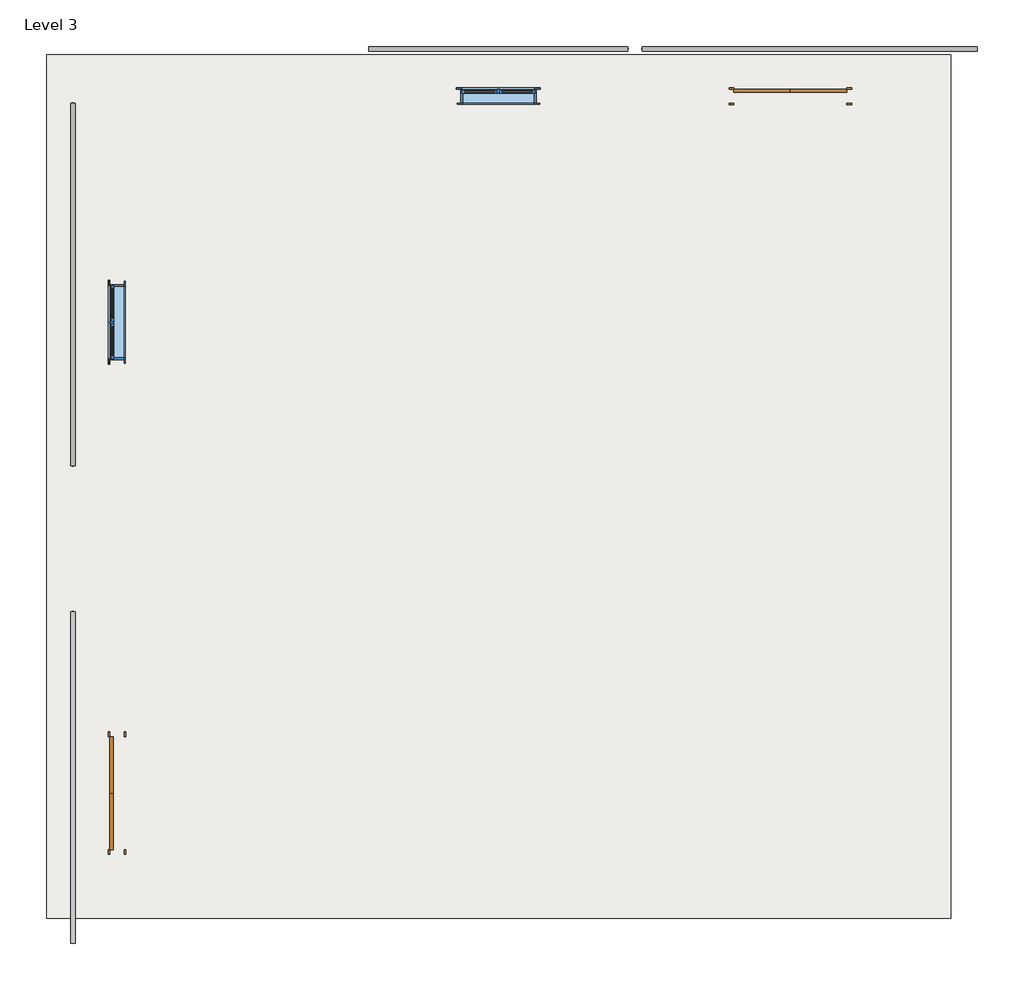
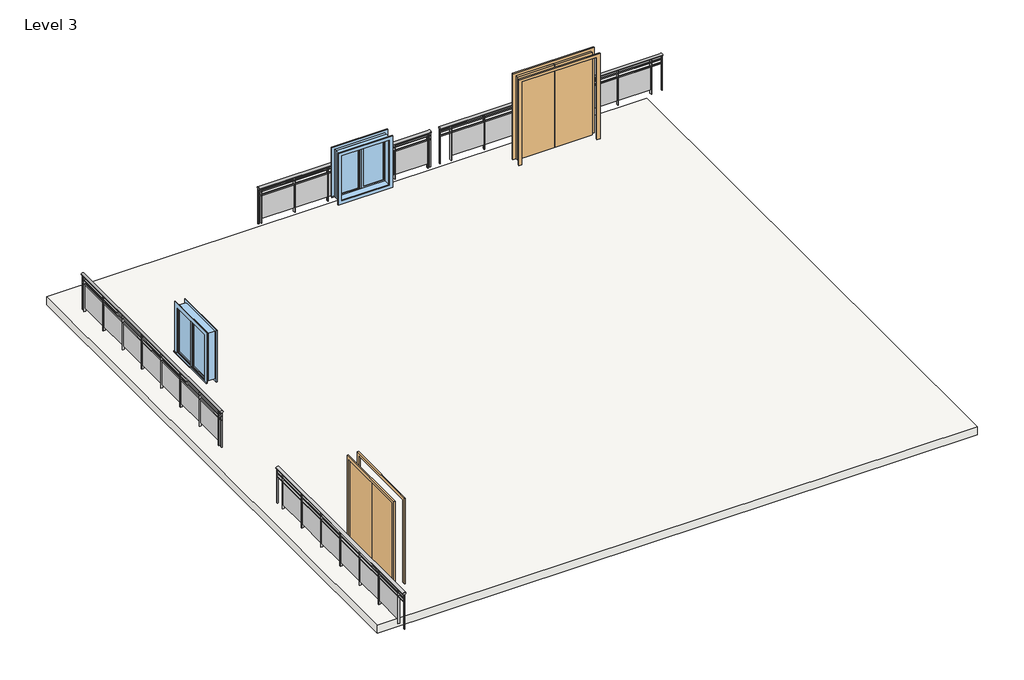
# One storey: 4 railings, 2 doors, 2 windows, 1 slab.
"""IFC4 building model written with IfcOpenShell, lengths in millimetres."""

from ifc_helpers import new_model, si_unit, point, frame, origin, place, context, project, spatial, polyline, ellipse_curve, trimmed, outline, extrude, transform, mapped, element, save
from ifc_brep_helpers import plane_surface, extruded_surface, advanced_brep
from components import door_640b4634, window_534dcd48

model = new_model("IFC4")

# Units and contexts
model_context = context("Model", 3, world=origin())
ifc_project = project(units=[si_unit("LENGTHUNIT", "METRE", prefix="MILLI")], contexts=[model_context])

# Site, building, storey
site = spatial("IfcSite", under=ifc_project)
building = spatial("IfcBuilding", under=site)
storey = spatial("IfcBuildingStorey", under=building, Name="Level 3", Elevation=6400.8)

# Doors
placement = place(None, origin())
door_shape = door_640b4634(model_context)
element("IfcDoor", 1, ObjectType="Door-Double-Flush_Panel : 72\" x 84\"", at=placement, inside=storey, context=model_context, shape_type="MappedRepresentation", body=[
    mapped(door_shape, transform((-18468.543393, -7089.1397804, 6400.8), x_axis=(0.0, 1.0, 0.0), y_axis=(-1.0, 0.0, 0.0), z_axis=(0.0, 0.0, 1.0))),
])
element("IfcDoor", 2, ObjectType="Door-Double-Flush_Panel : 72\" x 84\"", at=placement, inside=storey, context=model_context, shape_type="MappedRepresentation", body=[
    mapped(door_shape, transform((-7571.943393, 4188.4602196, 6400.8), x_axis=(1.0, 0.0, 0.0), y_axis=(0.0, 1.0, 0.0), z_axis=(0.0, 0.0, 1.0))),
])

# Railings
element("IfcRailing", 3, ObjectType="Glass Panel - Bottom Fill", at=placement, inside=storey, context=model_context, shape_type="SolidModel", body=[
    advanced_brep(
    [(-19220.0296876, -9514.8397804, 7315.2), (-19143.8296876, -9514.8397804, 7315.2), (-19220.0296876, -4155.4397804, 7315.2), (-19143.8296876, -4155.4397804, 7315.2)],
    [
        (0, 1, ellipse_curve(frame((-19181.9296876, -9514.8397804, 7315.2), z_axis=(0.0, -1.0, 0.0), x_axis=(1.0, 0.0, 0.0)), 38.1, 28.575)),
        (1, 0, ellipse_curve(frame((-19181.9296876, -9514.8397804, 7315.2), z_axis=(0.0, -1.0, 0.0), x_axis=(1.0, 0.0, 0.0)), 38.1, 28.575)),
        (2, 3, ellipse_curve(frame((-19181.9296876, -4155.4397804, 7315.2), z_axis=(0.0, 1.0, 0.0), x_axis=(1.0, 0.0, 0.0)), 38.1, 28.575)),
        (3, 2, ellipse_curve(frame((-19181.9296876, -4155.4397804, 7315.2), z_axis=(0.0, 1.0, 0.0), x_axis=(1.0, 0.0, 0.0)), 38.1, 28.575)),
        (0, 2),
        (3, 1),
    ],
    [
        plane_surface(frame((-19181.9296876, -9514.8397804, 7315.2), z_axis=(0.0, -1.0, 0.0), x_axis=(0.0, 0.0, 1.0))),
        plane_surface(frame((-19181.9296876, -4155.4397804, 7315.2), z_axis=(0.0, 1.0, 0.0), x_axis=(0.0, 0.0, 1.0))),
        extruded_surface(trimmed(ellipse_curve(frame((-19181.9296876, -4155.4397804, 7315.2), z_axis=(0.0, -1.0, 0.0), x_axis=(1.0, 0.0, 0.0)), 38.1, 28.575), [point((-19220.0296876, -4155.4397804, 7315.2))], [point((-19143.8296876, -4155.4397804, 7315.2))], True, "CARTESIAN"), (0.0, -5359.4, 0.0), 5359.4),
        extruded_surface(trimmed(ellipse_curve(frame((-19181.9296876, -4155.4397804, 7315.2), z_axis=(0.0, -1.0, 0.0), x_axis=(1.0, 0.0, 0.0)), 38.1, 28.575), [point((-19143.8296876, -4155.4397804, 7315.2))], [point((-19220.0296876, -4155.4397804, 7315.2))], True, "CARTESIAN"), (0.0, -5359.4, 0.0), 5359.4),
    ],
    [
        (0, [[1, 2]]),
        (1, [[3, 4]]),
        (2, [[-1, 5, -4, 6]]),
        (3, [[-2, -6, -3, -5]]),
    ],
),
    extrude(outline(polyline([(-19169.2296876, -9514.8397804), (-19194.6296876, -9514.8397804), (-19194.6296876, -4155.4397804), (-19169.2296876, -4155.4397804), (-19169.2296876, -9514.8397804)])), frame((0.0, 0.0, 7200.9), z_axis=(0.0, 0.0, 1.0), x_axis=(1.0, 0.0, 0.0)), (0.0, 0.0, 1.0), 25.4),
    extrude(outline(polyline([(-19169.2296876, -9514.8397804), (-19194.6296876, -9514.8397804), (-19194.6296876, -4155.4397804), (-19169.2296876, -4155.4397804), (-19169.2296876, -9514.8397804)])), frame((0.0, 0.0, 7099.3), z_axis=(0.0, 0.0, 1.0), x_axis=(1.0, 0.0, 0.0)), (0.0, 0.0, 1.0), 25.4),
    extrude(outline(polyline([(-19156.5296876, -4403.0897804), (-19207.3296876, -4403.0897804), (-19207.3296876, -4390.3897804), (-19156.5296876, -4390.3897804), (-19156.5296876, -4403.0897804)])), frame((0.0, 0.0, 6400.8), z_axis=(0.0, 0.0, 1.0), x_axis=(1.0, 0.0, 0.0)), (0.0, 0.0, 1.0), 885.6788223),
    extrude(outline(polyline([(-19188.4648446, -5209.5397804), (-19188.4648446, -4396.7397804), (-19182.1148446, -4396.7397804), (-19182.1148446, -5209.5397804), (-19188.4648446, -5209.5397804)])), frame((0.0, 0.0, 6502.4), z_axis=(0.0, 0.0, 1.0), x_axis=(1.0, 0.0, 0.0)), (0.0, 0.0, 1.0), 596.9),
    extrude(outline(polyline([(-19156.5296876, -5215.8897804), (-19207.3296876, -5215.8897804), (-19207.3296876, -5203.1897804), (-19156.5296876, -5203.1897804), (-19156.5296876, -5215.8897804)])), frame((0.0, 0.0, 6400.8), z_axis=(0.0, 0.0, 1.0), x_axis=(1.0, 0.0, 0.0)), (0.0, 0.0, 1.0), 885.6788223),
    extrude(outline(polyline([(-19188.4648446, -6022.3397804), (-19188.4648446, -5209.5397804), (-19182.1148446, -5209.5397804), (-19182.1148446, -6022.3397804), (-19188.4648446, -6022.3397804)])), frame((0.0, 0.0, 6502.4), z_axis=(0.0, 0.0, 1.0), x_axis=(1.0, 0.0, 0.0)), (0.0, 0.0, 1.0), 596.9),
    extrude(outline(polyline([(-19156.5296876, -6028.6897804), (-19207.3296876, -6028.6897804), (-19207.3296876, -6015.9897804), (-19156.5296876, -6015.9897804), (-19156.5296876, -6028.6897804)])), frame((0.0, 0.0, 6400.8), z_axis=(0.0, 0.0, 1.0), x_axis=(1.0, 0.0, 0.0)), (0.0, 0.0, 1.0), 885.6788223),
    extrude(outline(polyline([(-19188.4648446, -6835.1397804), (-19188.4648446, -6022.3397804), (-19182.1148446, -6022.3397804), (-19182.1148446, -6835.1397804), (-19188.4648446, -6835.1397804)])), frame((0.0, 0.0, 6502.4), z_axis=(0.0, 0.0, 1.0), x_axis=(1.0, 0.0, 0.0)), (0.0, 0.0, 1.0), 596.9),
    extrude(outline(polyline([(-19156.5296876, -6841.4897804), (-19207.3296876, -6841.4897804), (-19207.3296876, -6828.7897804), (-19156.5296876, -6828.7897804), (-19156.5296876, -6841.4897804)])), frame((0.0, 0.0, 6400.8), z_axis=(0.0, 0.0, 1.0), x_axis=(1.0, 0.0, 0.0)), (0.0, 0.0, 1.0), 885.6788223),
    extrude(outline(polyline([(-19188.4648446, -7647.9397804), (-19188.4648446, -6835.1397804), (-19182.1148446, -6835.1397804), (-19182.1148446, -7647.9397804), (-19188.4648446, -7647.9397804)])), frame((0.0, 0.0, 6502.4), z_axis=(0.0, 0.0, 1.0), x_axis=(1.0, 0.0, 0.0)), (0.0, 0.0, 1.0), 596.9),
    extrude(outline(polyline([(-19156.5296876, -7654.2897804), (-19207.3296876, -7654.2897804), (-19207.3296876, -7641.5897804), (-19156.5296876, -7641.5897804), (-19156.5296876, -7654.2897804)])), frame((0.0, 0.0, 6400.8), z_axis=(0.0, 0.0, 1.0), x_axis=(1.0, 0.0, 0.0)), (0.0, 0.0, 1.0), 885.6788223),
    extrude(outline(polyline([(-19188.4648446, -8460.7397804), (-19188.4648446, -7647.9397804), (-19182.1148446, -7647.9397804), (-19182.1148446, -8460.7397804), (-19188.4648446, -8460.7397804)])), frame((0.0, 0.0, 6502.4), z_axis=(0.0, 0.0, 1.0), x_axis=(1.0, 0.0, 0.0)), (0.0, 0.0, 1.0), 596.9),
    extrude(outline(polyline([(-19156.5296876, -8467.0897804), (-19207.3296876, -8467.0897804), (-19207.3296876, -8454.3897804), (-19156.5296876, -8454.3897804), (-19156.5296876, -8467.0897804)])), frame((0.0, 0.0, 6400.8), z_axis=(0.0, 0.0, 1.0), x_axis=(1.0, 0.0, 0.0)), (0.0, 0.0, 1.0), 885.6788223),
    extrude(outline(polyline([(-19188.4648446, -9273.5397804), (-19188.4648446, -8460.7397804), (-19182.1148446, -8460.7397804), (-19182.1148446, -9273.5397804), (-19188.4648446, -9273.5397804)])), frame((0.0, 0.0, 6502.4), z_axis=(0.0, 0.0, 1.0), x_axis=(1.0, 0.0, 0.0)), (0.0, 0.0, 1.0), 596.9),
    extrude(outline(polyline([(-19156.5296876, -9279.8897804), (-19207.3296876, -9279.8897804), (-19207.3296876, -9267.1897804), (-19156.5296876, -9267.1897804), (-19156.5296876, -9279.8897804)])), frame((0.0, 0.0, 6400.8), z_axis=(0.0, 0.0, 1.0), x_axis=(1.0, 0.0, 0.0)), (0.0, 0.0, 1.0), 885.6788223),
    extrude(outline(polyline([(-19172.4046876, -4168.1397804), (-19191.4546876, -4168.1397804), (-19191.4546876, -4149.0897804), (-19172.4046876, -4149.0897804), (-19172.4046876, -4168.1397804)])), frame((0.0, 0.0, 6400.8), z_axis=(0.0, 0.0, 1.0), x_axis=(1.0, 0.0, 0.0)), (0.0, 0.0, 1.0), 885.6788223),
    extrude(outline(polyline([(-19172.4046876, -9521.1897804), (-19191.4546876, -9521.1897804), (-19191.4546876, -9502.1397804), (-19172.4046876, -9502.1397804), (-19172.4046876, -9521.1897804)])), frame((0.0, 0.0, 6400.8), z_axis=(0.0, 0.0, 1.0), x_axis=(1.0, 0.0, 0.0)), (0.0, 0.0, 1.0), 885.6788223),
])
element("IfcRailing", 4, ObjectType="Glass Panel - Bottom Fill", at=placement, inside=storey, context=model_context, shape_type="SolidModel", body=[
    advanced_brep(
    [(-19143.8296876, 4074.1602196, 7315.2), (-19220.0296876, 4074.1602196, 7315.2), (-19143.8296876, -1793.2397804, 7315.2), (-19220.0296876, -1793.2397804, 7315.2)],
    [
        (0, 1, ellipse_curve(frame((-19181.9296876, 4074.1602196, 7315.2), z_axis=(0.0, 1.0, 0.0), x_axis=(-1.0, 0.0, 0.0)), 38.1, 28.575)),
        (1, 0, ellipse_curve(frame((-19181.9296876, 4074.1602196, 7315.2), z_axis=(0.0, 1.0, 0.0), x_axis=(-1.0, 0.0, 0.0)), 38.1, 28.575)),
        (2, 3, ellipse_curve(frame((-19181.9296876, -1793.2397804, 7315.2), z_axis=(0.0, -1.0, 0.0), x_axis=(-1.0, 0.0, 0.0)), 38.1, 28.575)),
        (3, 2, ellipse_curve(frame((-19181.9296876, -1793.2397804, 7315.2), z_axis=(0.0, -1.0, 0.0), x_axis=(-1.0, 0.0, 0.0)), 38.1, 28.575)),
        (0, 2),
        (3, 1),
    ],
    [
        plane_surface(frame((-19181.9296876, 4074.1602196, 7315.2), z_axis=(0.0, 1.0, 0.0), x_axis=(0.0, 0.0, -1.0))),
        plane_surface(frame((-19181.9296876, -1793.2397804, 7315.2), z_axis=(0.0, -1.0, 0.0), x_axis=(0.0, 0.0, -1.0))),
        extruded_surface(trimmed(ellipse_curve(frame((-19181.9296876, -1793.2397804, 7315.2), z_axis=(0.0, 1.0, 0.0), x_axis=(-1.0, 0.0, 0.0)), 38.1, 28.575), [point((-19143.8296876, -1793.2397804, 7315.2))], [point((-19220.0296876, -1793.2397804, 7315.2))], True, "CARTESIAN"), (0.0, 5867.4, 0.0), 5867.4),
        extruded_surface(trimmed(ellipse_curve(frame((-19181.9296876, -1793.2397804, 7315.2), z_axis=(0.0, 1.0, 0.0), x_axis=(-1.0, 0.0, 0.0)), 38.1, 28.575), [point((-19220.0296876, -1793.2397804, 7315.2))], [point((-19143.8296876, -1793.2397804, 7315.2))], True, "CARTESIAN"), (0.0, 5867.4, 0.0), 5867.4),
    ],
    [
        (0, [[1, 2]]),
        (1, [[3, 4]]),
        (2, [[-1, 5, -4, 6]]),
        (3, [[-2, -6, -3, -5]]),
    ],
),
    extrude(outline(polyline([(-19194.6296876, 4074.1602196), (-19169.2296876, 4074.1602196), (-19169.2296876, -1793.2397804), (-19194.6296876, -1793.2397804), (-19194.6296876, 4074.1602196)])), frame((0.0, 0.0, 7200.9), z_axis=(0.0, 0.0, 1.0), x_axis=(1.0, 0.0, 0.0)), (0.0, 0.0, 1.0), 25.4),
    extrude(outline(polyline([(-19194.6296876, 4074.1602196), (-19169.2296876, 4074.1602196), (-19169.2296876, -1793.2397804), (-19194.6296876, -1793.2397804), (-19194.6296876, 4074.1602196)])), frame((0.0, 0.0, 7099.3), z_axis=(0.0, 0.0, 1.0), x_axis=(1.0, 0.0, 0.0)), (0.0, 0.0, 1.0), 25.4),
    extrude(outline(polyline([(-19207.3296876, -1697.9897804), (-19156.5296876, -1697.9897804), (-19156.5296876, -1710.6897804), (-19207.3296876, -1710.6897804), (-19207.3296876, -1697.9897804)])), frame((0.0, 0.0, 6400.8), z_axis=(0.0, 0.0, 1.0), x_axis=(1.0, 0.0, 0.0)), (0.0, 0.0, 1.0), 885.6788223),
    extrude(outline(polyline([(-19175.3945306, -891.5397804), (-19175.3945306, -1704.3397804), (-19181.7445306, -1704.3397804), (-19181.7445306, -891.5397804), (-19175.3945306, -891.5397804)])), frame((0.0, 0.0, 6502.4), z_axis=(0.0, 0.0, 1.0), x_axis=(1.0, 0.0, 0.0)), (0.0, 0.0, 1.0), 596.9),
    extrude(outline(polyline([(-19207.3296876, -885.1897804), (-19156.5296876, -885.1897804), (-19156.5296876, -897.8897804), (-19207.3296876, -897.8897804), (-19207.3296876, -885.1897804)])), frame((0.0, 0.0, 6400.8), z_axis=(0.0, 0.0, 1.0), x_axis=(1.0, 0.0, 0.0)), (0.0, 0.0, 1.0), 885.6788223),
    extrude(outline(polyline([(-19175.3945306, -78.7397804), (-19175.3945306, -891.5397804), (-19181.7445306, -891.5397804), (-19181.7445306, -78.7397804), (-19175.3945306, -78.7397804)])), frame((0.0, 0.0, 6502.4), z_axis=(0.0, 0.0, 1.0), x_axis=(1.0, 0.0, 0.0)), (0.0, 0.0, 1.0), 596.9),
    extrude(outline(polyline([(-19207.3296876, -72.3897804), (-19156.5296876, -72.3897804), (-19156.5296876, -85.0897804), (-19207.3296876, -85.0897804), (-19207.3296876, -72.3897804)])), frame((0.0, 0.0, 6400.8), z_axis=(0.0, 0.0, 1.0), x_axis=(1.0, 0.0, 0.0)), (0.0, 0.0, 1.0), 885.6788223),
    extrude(outline(polyline([(-19175.3945306, 734.0602196), (-19175.3945306, -78.7397804), (-19181.7445306, -78.7397804), (-19181.7445306, 734.0602196), (-19175.3945306, 734.0602196)])), frame((0.0, 0.0, 6502.4), z_axis=(0.0, 0.0, 1.0), x_axis=(1.0, 0.0, 0.0)), (0.0, 0.0, 1.0), 596.9),
    extrude(outline(polyline([(-19207.3296876, 740.4102196), (-19156.5296876, 740.4102196), (-19156.5296876, 727.7102196), (-19207.3296876, 727.7102196), (-19207.3296876, 740.4102196)])), frame((0.0, 0.0, 6400.8), z_axis=(0.0, 0.0, 1.0), x_axis=(1.0, 0.0, 0.0)), (0.0, 0.0, 1.0), 885.6788223),
    extrude(outline(polyline([(-19175.3945306, 1546.8602196), (-19175.3945306, 734.0602196), (-19181.7445306, 734.0602196), (-19181.7445306, 1546.8602196), (-19175.3945306, 1546.8602196)])), frame((0.0, 0.0, 6502.4), z_axis=(0.0, 0.0, 1.0), x_axis=(1.0, 0.0, 0.0)), (0.0, 0.0, 1.0), 596.9),
    extrude(outline(polyline([(-19207.3296876, 1553.2102196), (-19156.5296876, 1553.2102196), (-19156.5296876, 1540.5102196), (-19207.3296876, 1540.5102196), (-19207.3296876, 1553.2102196)])), frame((0.0, 0.0, 6400.8), z_axis=(0.0, 0.0, 1.0), x_axis=(1.0, 0.0, 0.0)), (0.0, 0.0, 1.0), 885.6788223),
    extrude(outline(polyline([(-19175.3945306, 2359.6602196), (-19175.3945306, 1546.8602196), (-19181.7445306, 1546.8602196), (-19181.7445306, 2359.6602196), (-19175.3945306, 2359.6602196)])), frame((0.0, 0.0, 6502.4), z_axis=(0.0, 0.0, 1.0), x_axis=(1.0, 0.0, 0.0)), (0.0, 0.0, 1.0), 596.9),
    extrude(outline(polyline([(-19207.3296876, 2366.0102196), (-19156.5296876, 2366.0102196), (-19156.5296876, 2353.3102196), (-19207.3296876, 2353.3102196), (-19207.3296876, 2366.0102196)])), frame((0.0, 0.0, 6400.8), z_axis=(0.0, 0.0, 1.0), x_axis=(1.0, 0.0, 0.0)), (0.0, 0.0, 1.0), 885.6788223),
    extrude(outline(polyline([(-19175.3945306, 3172.4602196), (-19175.3945306, 2359.6602196), (-19181.7445306, 2359.6602196), (-19181.7445306, 3172.4602196), (-19175.3945306, 3172.4602196)])), frame((0.0, 0.0, 6502.4), z_axis=(0.0, 0.0, 1.0), x_axis=(1.0, 0.0, 0.0)), (0.0, 0.0, 1.0), 596.9),
    extrude(outline(polyline([(-19207.3296876, 3178.8102196), (-19156.5296876, 3178.8102196), (-19156.5296876, 3166.1102196), (-19207.3296876, 3166.1102196), (-19207.3296876, 3178.8102196)])), frame((0.0, 0.0, 6400.8), z_axis=(0.0, 0.0, 1.0), x_axis=(1.0, 0.0, 0.0)), (0.0, 0.0, 1.0), 885.6788223),
    extrude(outline(polyline([(-19175.3945306, 3985.2602196), (-19175.3945306, 3172.4602196), (-19181.7445306, 3172.4602196), (-19181.7445306, 3985.2602196), (-19175.3945306, 3985.2602196)])), frame((0.0, 0.0, 6502.4), z_axis=(0.0, 0.0, 1.0), x_axis=(1.0, 0.0, 0.0)), (0.0, 0.0, 1.0), 596.9),
    extrude(outline(polyline([(-19207.3296876, 3991.6102196), (-19156.5296876, 3991.6102196), (-19156.5296876, 3978.9102196), (-19207.3296876, 3978.9102196), (-19207.3296876, 3991.6102196)])), frame((0.0, 0.0, 6400.8), z_axis=(0.0, 0.0, 1.0), x_axis=(1.0, 0.0, 0.0)), (0.0, 0.0, 1.0), 885.6788223),
    extrude(outline(polyline([(-19191.4546876, -1780.5397804), (-19172.4046876, -1780.5397804), (-19172.4046876, -1799.5897804), (-19191.4546876, -1799.5897804), (-19191.4546876, -1780.5397804)])), frame((0.0, 0.0, 6400.8), z_axis=(0.0, 0.0, 1.0), x_axis=(1.0, 0.0, 0.0)), (0.0, 0.0, 1.0), 885.6788223),
    extrude(outline(polyline([(-19191.4546876, 4080.5102196), (-19172.4046876, 4080.5102196), (-19172.4046876, 4061.4602196), (-19191.4546876, 4061.4602196), (-19191.4546876, 4080.5102196)])), frame((0.0, 0.0, 6400.8), z_axis=(0.0, 0.0, 1.0), x_axis=(1.0, 0.0, 0.0)), (0.0, 0.0, 1.0), 885.6788223),
])
element("IfcRailing", 5, ObjectType="Glass Panel - Bottom Fill", at=placement, inside=storey, context=model_context, shape_type="SolidModel", body=[
    advanced_brep(
    [(-14391.843393, 4991.4940048, 7315.2), (-14391.843393, 4915.2940048, 7315.2), (-10200.843393, 4991.4940048, 7315.2), (-10200.843393, 4915.2940048, 7315.2)],
    [
        (0, 1, ellipse_curve(frame((-14391.843393, 4953.3940048, 7315.2), z_axis=(-1.0, 0.0, 0.0), x_axis=(0.0, -1.0, 0.0)), 38.1, 28.575)),
        (1, 0, ellipse_curve(frame((-14391.843393, 4953.3940048, 7315.2), z_axis=(-1.0, 0.0, 0.0), x_axis=(0.0, -1.0, 0.0)), 38.1, 28.575)),
        (2, 3, ellipse_curve(frame((-10200.843393, 4953.3940048, 7315.2), z_axis=(1.0, 0.0, 0.0), x_axis=(0.0, -1.0, 0.0)), 38.1, 28.575)),
        (3, 2, ellipse_curve(frame((-10200.843393, 4953.3940048, 7315.2), z_axis=(1.0, 0.0, 0.0), x_axis=(0.0, -1.0, 0.0)), 38.1, 28.575)),
        (0, 2),
        (3, 1),
    ],
    [
        plane_surface(frame((-14391.843393, 4953.3940048, 7315.2), z_axis=(-1.0, 0.0, 0.0), x_axis=(0.0, 1.0, 0.0))),
        plane_surface(frame((-10200.843393, 4953.3940048, 7315.2), z_axis=(1.0, 0.0, 0.0), x_axis=(0.0, 1.0, 0.0))),
        extruded_surface(trimmed(ellipse_curve(frame((-10200.843393, 4953.3940048, 7315.2), z_axis=(-1.0, 0.0, 0.0), x_axis=(0.0, -1.0, 0.0)), 38.1, 28.575), [point((-10200.843393, 4991.4940048, 7315.2))], [point((-10200.843393, 4915.2940048, 7315.2))], True, "CARTESIAN"), (-4191.0, 0.0, 0.0), 4191.0),
        extruded_surface(trimmed(ellipse_curve(frame((-10200.843393, 4953.3940048, 7315.2), z_axis=(-1.0, 0.0, 0.0), x_axis=(0.0, -1.0, 0.0)), 38.1, 28.575), [point((-10200.843393, 4915.2940048, 7315.2))], [point((-10200.843393, 4991.4940048, 7315.2))], True, "CARTESIAN"), (-4191.0, 0.0, 0.0), 4191.0),
    ],
    [
        (0, [[1, 2]]),
        (1, [[3, 4]]),
        (2, [[-1, 5, -4, 6]]),
        (3, [[-2, -6, -3, -5]]),
    ],
),
    extrude(outline(polyline([(-14391.843393, 4940.6940048), (-14391.843393, 4966.0940048), (-10200.843393, 4966.0940048), (-10200.843393, 4940.6940048), (-14391.843393, 4940.6940048)])), frame((0.0, 0.0, 7200.9), z_axis=(0.0, 0.0, 1.0), x_axis=(1.0, 0.0, 0.0)), (0.0, 0.0, 1.0), 25.4),
    extrude(outline(polyline([(-14391.843393, 4940.6940048), (-14391.843393, 4966.0940048), (-10200.843393, 4966.0940048), (-10200.843393, 4940.6940048), (-14391.843393, 4940.6940048)])), frame((0.0, 0.0, 7099.3), z_axis=(0.0, 0.0, 1.0), x_axis=(1.0, 0.0, 0.0)), (0.0, 0.0, 1.0), 25.4),
    extrude(outline(polyline([(-10270.693393, 4927.9940048), (-10270.693393, 4978.7940048), (-10257.993393, 4978.7940048), (-10257.993393, 4927.9940048), (-10270.693393, 4927.9940048)])), frame((0.0, 0.0, 6400.8), z_axis=(0.0, 0.0, 1.0), x_axis=(1.0, 0.0, 0.0)), (0.0, 0.0, 1.0), 885.6788223),
    extrude(outline(polyline([(-11077.143393, 4959.9291618), (-10264.343393, 4959.9291618), (-10264.343393, 4953.5791618), (-11077.143393, 4953.5791618), (-11077.143393, 4959.9291618)])), frame((0.0, 0.0, 6502.4), z_axis=(0.0, 0.0, 1.0), x_axis=(1.0, 0.0, 0.0)), (0.0, 0.0, 1.0), 596.9),
    extrude(outline(polyline([(-11083.493393, 4927.9940048), (-11083.493393, 4978.7940048), (-11070.793393, 4978.7940048), (-11070.793393, 4927.9940048), (-11083.493393, 4927.9940048)])), frame((0.0, 0.0, 6400.8), z_axis=(0.0, 0.0, 1.0), x_axis=(1.0, 0.0, 0.0)), (0.0, 0.0, 1.0), 885.6788223),
    extrude(outline(polyline([(-11889.943393, 4959.9291618), (-11077.143393, 4959.9291618), (-11077.143393, 4953.5791618), (-11889.943393, 4953.5791618), (-11889.943393, 4959.9291618)])), frame((0.0, 0.0, 6502.4), z_axis=(0.0, 0.0, 1.0), x_axis=(1.0, 0.0, 0.0)), (0.0, 0.0, 1.0), 596.9),
    extrude(outline(polyline([(-11896.293393, 4927.9940048), (-11896.293393, 4978.7940048), (-11883.593393, 4978.7940048), (-11883.593393, 4927.9940048), (-11896.293393, 4927.9940048)])), frame((0.0, 0.0, 6400.8), z_axis=(0.0, 0.0, 1.0), x_axis=(1.0, 0.0, 0.0)), (0.0, 0.0, 1.0), 885.6788223),
    extrude(outline(polyline([(-12702.743393, 4959.9291618), (-11889.943393, 4959.9291618), (-11889.943393, 4953.5791618), (-12702.743393, 4953.5791618), (-12702.743393, 4959.9291618)])), frame((0.0, 0.0, 6502.4), z_axis=(0.0, 0.0, 1.0), x_axis=(1.0, 0.0, 0.0)), (0.0, 0.0, 1.0), 596.9),
    extrude(outline(polyline([(-12709.093393, 4927.9940048), (-12709.093393, 4978.7940048), (-12696.393393, 4978.7940048), (-12696.393393, 4927.9940048), (-12709.093393, 4927.9940048)])), frame((0.0, 0.0, 6400.8), z_axis=(0.0, 0.0, 1.0), x_axis=(1.0, 0.0, 0.0)), (0.0, 0.0, 1.0), 885.6788223),
    extrude(outline(polyline([(-13515.543393, 4959.9291618), (-12702.743393, 4959.9291618), (-12702.743393, 4953.5791618), (-13515.543393, 4953.5791618), (-13515.543393, 4959.9291618)])), frame((0.0, 0.0, 6502.4), z_axis=(0.0, 0.0, 1.0), x_axis=(1.0, 0.0, 0.0)), (0.0, 0.0, 1.0), 596.9),
    extrude(outline(polyline([(-13521.893393, 4927.9940048), (-13521.893393, 4978.7940048), (-13509.193393, 4978.7940048), (-13509.193393, 4927.9940048), (-13521.893393, 4927.9940048)])), frame((0.0, 0.0, 6400.8), z_axis=(0.0, 0.0, 1.0), x_axis=(1.0, 0.0, 0.0)), (0.0, 0.0, 1.0), 885.6788223),
    extrude(outline(polyline([(-14328.343393, 4959.9291618), (-13515.543393, 4959.9291618), (-13515.543393, 4953.5791618), (-14328.343393, 4953.5791618), (-14328.343393, 4959.9291618)])), frame((0.0, 0.0, 6502.4), z_axis=(0.0, 0.0, 1.0), x_axis=(1.0, 0.0, 0.0)), (0.0, 0.0, 1.0), 596.9),
    extrude(outline(polyline([(-14334.693393, 4927.9940048), (-14334.693393, 4978.7940048), (-14321.993393, 4978.7940048), (-14321.993393, 4927.9940048), (-14334.693393, 4927.9940048)])), frame((0.0, 0.0, 6400.8), z_axis=(0.0, 0.0, 1.0), x_axis=(1.0, 0.0, 0.0)), (0.0, 0.0, 1.0), 885.6788223),
    extrude(outline(polyline([(-10213.543393, 4943.8690048), (-10213.543393, 4962.9190048), (-10194.493393, 4962.9190048), (-10194.493393, 4943.8690048), (-10213.543393, 4943.8690048)])), frame((0.0, 0.0, 6400.8), z_axis=(0.0, 0.0, 1.0), x_axis=(1.0, 0.0, 0.0)), (0.0, 0.0, 1.0), 885.6788223),
    extrude(outline(polyline([(-14398.193393, 4943.8690048), (-14398.193393, 4962.9190048), (-14379.143393, 4962.9190048), (-14379.143393, 4943.8690048), (-14398.193393, 4943.8690048)])), frame((0.0, 0.0, 6400.8), z_axis=(0.0, 0.0, 1.0), x_axis=(1.0, 0.0, 0.0)), (0.0, 0.0, 1.0), 885.6788223),
])
element("IfcRailing", 6, ObjectType="Glass Panel - Bottom Fill", at=placement, inside=storey, context=model_context, shape_type="SolidModel", body=[
    advanced_brep(
    [(-9972.243393, 4991.4940048, 7315.2), (-9972.243393, 4915.2940048, 7315.2), (-4551.5296876, 4991.4940048, 7315.2), (-4551.5296876, 4915.2940048, 7315.2)],
    [
        (0, 1, ellipse_curve(frame((-9972.243393, 4953.3940048, 7315.2), z_axis=(-1.0, 0.0, 0.0), x_axis=(0.0, -1.0, 0.0)), 38.1, 28.575)),
        (1, 0, ellipse_curve(frame((-9972.243393, 4953.3940048, 7315.2), z_axis=(-1.0, 0.0, 0.0), x_axis=(0.0, -1.0, 0.0)), 38.1, 28.575)),
        (2, 3, ellipse_curve(frame((-4551.5296876, 4953.3940048, 7315.2), z_axis=(1.0, 0.0, 0.0), x_axis=(0.0, -1.0, 0.0)), 38.1, 28.575)),
        (3, 2, ellipse_curve(frame((-4551.5296876, 4953.3940048, 7315.2), z_axis=(1.0, 0.0, 0.0), x_axis=(0.0, -1.0, 0.0)), 38.1, 28.575)),
        (0, 2),
        (3, 1),
    ],
    [
        plane_surface(frame((-9972.243393, 4953.3940048, 7315.2), z_axis=(-1.0, 0.0, 0.0), x_axis=(0.0, 1.0, 0.0))),
        plane_surface(frame((-4551.5296876, 4953.3940048, 7315.2), z_axis=(1.0, 0.0, 0.0), x_axis=(0.0, 1.0, 0.0))),
        extruded_surface(trimmed(ellipse_curve(frame((-4551.5296876, 4953.3940048, 7315.2), z_axis=(-1.0, 0.0, 0.0), x_axis=(0.0, -1.0, 0.0)), 38.1, 28.575), [point((-4551.5296876, 4991.4940048, 7315.2))], [point((-4551.5296876, 4915.2940048, 7315.2))], True, "CARTESIAN"), (-5420.7137054, 0.0, 0.0), 5420.7137054),
        extruded_surface(trimmed(ellipse_curve(frame((-4551.5296876, 4953.3940048, 7315.2), z_axis=(-1.0, 0.0, 0.0), x_axis=(0.0, -1.0, 0.0)), 38.1, 28.575), [point((-4551.5296876, 4915.2940048, 7315.2))], [point((-4551.5296876, 4991.4940048, 7315.2))], True, "CARTESIAN"), (-5420.7137054, 0.0, 0.0), 5420.7137054),
    ],
    [
        (0, [[1, 2]]),
        (1, [[3, 4]]),
        (2, [[-1, 5, -4, 6]]),
        (3, [[-2, -6, -3, -5]]),
    ],
),
    extrude(outline(polyline([(-9972.243393, 4940.6940048), (-9972.243393, 4966.0940048), (-4551.5296876, 4966.0940048), (-4551.5296876, 4940.6940048), (-9972.243393, 4940.6940048)])), frame((0.0, 0.0, 7200.9), z_axis=(0.0, 0.0, 1.0), x_axis=(1.0, 0.0, 0.0)), (0.0, 0.0, 1.0), 25.4),
    extrude(outline(polyline([(-9972.243393, 4940.6940048), (-9972.243393, 4966.0940048), (-4551.5296876, 4966.0940048), (-4551.5296876, 4940.6940048), (-9972.243393, 4940.6940048)])), frame((0.0, 0.0, 7099.3), z_axis=(0.0, 0.0, 1.0), x_axis=(1.0, 0.0, 0.0)), (0.0, 0.0, 1.0), 25.4),
    extrude(outline(polyline([(-4829.8365403, 4927.9940048), (-4829.8365403, 4978.7940048), (-4817.1365403, 4978.7940048), (-4817.1365403, 4927.9940048), (-4829.8365403, 4927.9940048)])), frame((0.0, 0.0, 6400.8), z_axis=(0.0, 0.0, 1.0), x_axis=(1.0, 0.0, 0.0)), (0.0, 0.0, 1.0), 885.6788223),
    extrude(outline(polyline([(-5636.2865403, 4959.9291618), (-4823.4865403, 4959.9291618), (-4823.4865403, 4953.5791618), (-5636.2865403, 4953.5791618), (-5636.2865403, 4959.9291618)])), frame((0.0, 0.0, 6502.4), z_axis=(0.0, 0.0, 1.0), x_axis=(1.0, 0.0, 0.0)), (0.0, 0.0, 1.0), 596.9),
    extrude(outline(polyline([(-5642.6365403, 4927.9940048), (-5642.6365403, 4978.7940048), (-5629.9365403, 4978.7940048), (-5629.9365403, 4927.9940048), (-5642.6365403, 4927.9940048)])), frame((0.0, 0.0, 6400.8), z_axis=(0.0, 0.0, 1.0), x_axis=(1.0, 0.0, 0.0)), (0.0, 0.0, 1.0), 885.6788223),
    extrude(outline(polyline([(-6449.0865403, 4959.9291618), (-5636.2865403, 4959.9291618), (-5636.2865403, 4953.5791618), (-6449.0865403, 4953.5791618), (-6449.0865403, 4959.9291618)])), frame((0.0, 0.0, 6502.4), z_axis=(0.0, 0.0, 1.0), x_axis=(1.0, 0.0, 0.0)), (0.0, 0.0, 1.0), 596.9),
    extrude(outline(polyline([(-6455.4365403, 4927.9940048), (-6455.4365403, 4978.7940048), (-6442.7365403, 4978.7940048), (-6442.7365403, 4927.9940048), (-6455.4365403, 4927.9940048)])), frame((0.0, 0.0, 6400.8), z_axis=(0.0, 0.0, 1.0), x_axis=(1.0, 0.0, 0.0)), (0.0, 0.0, 1.0), 885.6788223),
    extrude(outline(polyline([(-7261.8865403, 4959.9291618), (-6449.0865403, 4959.9291618), (-6449.0865403, 4953.5791618), (-7261.8865403, 4953.5791618), (-7261.8865403, 4959.9291618)])), frame((0.0, 0.0, 6502.4), z_axis=(0.0, 0.0, 1.0), x_axis=(1.0, 0.0, 0.0)), (0.0, 0.0, 1.0), 596.9),
    extrude(outline(polyline([(-7268.2365403, 4927.9940048), (-7268.2365403, 4978.7940048), (-7255.5365403, 4978.7940048), (-7255.5365403, 4927.9940048), (-7268.2365403, 4927.9940048)])), frame((0.0, 0.0, 6400.8), z_axis=(0.0, 0.0, 1.0), x_axis=(1.0, 0.0, 0.0)), (0.0, 0.0, 1.0), 885.6788223),
    extrude(outline(polyline([(-8074.6865403, 4959.9291618), (-7261.8865403, 4959.9291618), (-7261.8865403, 4953.5791618), (-8074.6865403, 4953.5791618), (-8074.6865403, 4959.9291618)])), frame((0.0, 0.0, 6502.4), z_axis=(0.0, 0.0, 1.0), x_axis=(1.0, 0.0, 0.0)), (0.0, 0.0, 1.0), 596.9),
    extrude(outline(polyline([(-8081.0365403, 4927.9940048), (-8081.0365403, 4978.7940048), (-8068.3365403, 4978.7940048), (-8068.3365403, 4927.9940048), (-8081.0365403, 4927.9940048)])), frame((0.0, 0.0, 6400.8), z_axis=(0.0, 0.0, 1.0), x_axis=(1.0, 0.0, 0.0)), (0.0, 0.0, 1.0), 885.6788223),
    extrude(outline(polyline([(-8887.4865403, 4959.9291618), (-8074.6865403, 4959.9291618), (-8074.6865403, 4953.5791618), (-8887.4865403, 4953.5791618), (-8887.4865403, 4959.9291618)])), frame((0.0, 0.0, 6502.4), z_axis=(0.0, 0.0, 1.0), x_axis=(1.0, 0.0, 0.0)), (0.0, 0.0, 1.0), 596.9),
    extrude(outline(polyline([(-8893.8365403, 4927.9940048), (-8893.8365403, 4978.7940048), (-8881.1365403, 4978.7940048), (-8881.1365403, 4927.9940048), (-8893.8365403, 4927.9940048)])), frame((0.0, 0.0, 6400.8), z_axis=(0.0, 0.0, 1.0), x_axis=(1.0, 0.0, 0.0)), (0.0, 0.0, 1.0), 885.6788223),
    extrude(outline(polyline([(-9700.2865403, 4959.9291618), (-8887.4865403, 4959.9291618), (-8887.4865403, 4953.5791618), (-9700.2865403, 4953.5791618), (-9700.2865403, 4959.9291618)])), frame((0.0, 0.0, 6502.4), z_axis=(0.0, 0.0, 1.0), x_axis=(1.0, 0.0, 0.0)), (0.0, 0.0, 1.0), 596.9),
    extrude(outline(polyline([(-9706.6365403, 4927.9940048), (-9706.6365403, 4978.7940048), (-9693.9365403, 4978.7940048), (-9693.9365403, 4927.9940048), (-9706.6365403, 4927.9940048)])), frame((0.0, 0.0, 6400.8), z_axis=(0.0, 0.0, 1.0), x_axis=(1.0, 0.0, 0.0)), (0.0, 0.0, 1.0), 885.6788223),
    extrude(outline(polyline([(-4564.2296876, 4943.8690048), (-4564.2296876, 4962.9190048), (-4545.1796876, 4962.9190048), (-4545.1796876, 4943.8690048), (-4564.2296876, 4943.8690048)])), frame((0.0, 0.0, 6400.8), z_axis=(0.0, 0.0, 1.0), x_axis=(1.0, 0.0, 0.0)), (0.0, 0.0, 1.0), 885.6788223),
    extrude(outline(polyline([(-9978.593393, 4943.8690048), (-9978.593393, 4962.9190048), (-9959.543393, 4962.9190048), (-9959.543393, 4943.8690048), (-9978.593393, 4943.8690048)])), frame((0.0, 0.0, 6400.8), z_axis=(0.0, 0.0, 1.0), x_axis=(1.0, 0.0, 0.0)), (0.0, 0.0, 1.0), 885.6788223),
])

# Slab
element("IfcSlab", 7, ObjectType="Generic - 12\"", at=placement, inside=storey, context=model_context, shape_type="SweptSolid", body=[
    extrude(outline(polyline([(-4978.1294205, 4859.2425906), (-4978.1294205, -9111.9352984), (-19608.5294205, -9111.9352984), (-19608.5294205, 4859.2425906), (-4978.1294205, 4859.2425906)])), frame((0.0, 0.0, 6197.6), z_axis=(0.0, 0.0, 1.0), x_axis=(1.0, 0.0, 0.0)), (0.0, 0.0, 1.0), 203.2),
])

# Windows
window_shape = window_534dcd48(model_context)
element("IfcWindow", 8, ObjectType="Casement Dbl with Trim : 48\" x 48\"", at=placement, inside=storey, context=model_context, shape_type="MappedRepresentation", body=[
    mapped(window_shape, transform((-18449.493393, 530.8602196, 5933.0186704), x_axis=(0.0, 1.0, 0.0), y_axis=(-1.0, 0.0, 0.0), z_axis=(0.0, 0.0, 1.0))),
])
element("IfcWindow", 9, ObjectType="Casement Dbl with Trim : 48\" x 48\"", at=placement, inside=storey, context=model_context, shape_type="MappedRepresentation", body=[
    mapped(window_shape, transform((-12296.343393, 4169.4102196, 6058.2927979), x_axis=(1.0, 0.0, 0.0), y_axis=(0.0, 1.0, 0.0), z_axis=(0.0, 0.0, 1.0))),
])

save(model, "model.ifc")

# Revit data of these elements
# Type "Door-Double-Flush_Panel : 72\" x 84\""
#   Type Mark = "11"
#   Construction Type Id = "DOOR"
#   Assembly Code = "C1020"
#   Analytic Construction = "Wooden"
#   Thickness = 0' - 2"
#   Thermal Resistance (R) = 2.5876 (h·ft²·°F)/BTU
#   Swing Angle [instance default] = 90.00°
#   Panel Width = 3' - 0"
#   Heat Transfer Coefficient (U) = 0.3865 BTU/(h·ft²·°F)
#   Height = 7' - 0"
#   Trim Projection Ext = 0' - 1"
#   Trim Projection Int = 0' - 1"
#   Trim Width = 0' - 3"
#   Width = 6' - 0"
#   Define Thermal Properties by = 1
#   Panel Material = Glass, Clear Glazing
#   Trim Material = Paint - Sienna
#   Visual Light Transmittance = 0
#   Solar Heat Gain Coefficient = 0
#   Function = (empty or 0)
#   Wall Closure = (empty or 0)
# Type "Glass Panel - Bottom Fill"
#   Assembly Code = "C2010400"
#   built-in parameter 1008612 = 0.0416667 (stored number, unit not read)
#   built-in parameter 1008611 = 0.0416667 (stored number, unit not read)
#   built-in parameter 1008609 = 0.333333 (stored number, unit not read)
#   built-in parameter 1008604 = 0.166667 (stored number, unit not read)
#   built-in parameter 1008603 = 0.166667 (stored number, unit not read)
#   Railing Height = 3' - 0"
#   built-in parameter 1008630 = 2
#   built-in parameter 1008610 = 2
#   built-in parameter 1008618 = Baluster - Square : 3/4"
# Type "Generic - 12\""
#   Assembly Code = "B1010"
#   Function = 0
#   Layers, outside or top first: 0' - 8" no material (function 1)
# Type "Casement Dbl with Trim : 48\" x 48\""
#   Type Mark = "10"
#   Construction Type Id = "GSP4R"
#   Assembly Code = "B2020100"
#   Analytic Construction = "1/8 in Pilkington single glazing"
#   Visual Light Transmittance = 0.9
#   Solar Heat Gain Coefficient = 0.78
#   Heat Transfer Coefficient (U) = 0.6496 BTU/(h·ft²·°F)
#   Height = 4' - 0"
#   Default Sill Height = 3' - 0"
#   Trim Projection - Ext. = 0' - 0 1/2"
#   Trim Projection - Int. = 0' - 0 3/4"
#   Trim Width - Exterior = 0' - 3 1/2"
#   Trim Width - Interior = 0' - 3 1/2"
#   Width = 4' - 0"
#   Window Inset = 0' - 0 3/4"
#   Define Thermal Properties by = 1
#   Glass Pane Material = Glass
#   Sash Material = Glass, Clear Glazing
#   Trim Exterior Material = Earth
#   Trim Interior Material = Trim
#   Wall Closure = (empty or 0)
# Elements 1, 2 (IfcDoor, "Door-Double-Flush_Panel : 72\" x 84\"")
#   Swing Angle = 90.00°
#   Phase Created = New Construction
#   Materials on its faces: "Paint - Sienna", "Glass, Clear Glazing"
# Elements 3, 4, 5, 6 (IfcRailing, "Glass Panel - Bottom Fill")
#   Phase Created = New Construction
#   Materials on its faces: "Glass"
# Element 7 (IfcSlab, "Generic - 12\"")
#   Height Offset From Level = 0' - 0"
#   Phase Created = New Construction
#   Materials on its faces: "Default Floor"
# Element 8 (IfcWindow, "Casement Dbl with Trim : 48\" x 48\"")
#   Mark = "2"
#   Phase Created = New Construction
#   Materials on its faces: "Glass, Clear Glazing", "Earth", "Glass", "Trim"
# Element 9 (IfcWindow, "Casement Dbl with Trim : 48\" x 48\"")
#   Mark = "7"
#   Phase Created = New Construction
#   Materials on its faces: "Glass, Clear Glazing", "Earth", "Glass", "Trim"
# Materials
#   "Glass, Clear Glazing": class "Glass", colour RGB 0 128 192, transparency 0.75, Description = "Clear glazing", Cost = 0
#   "Paint - Sienna": colour RGB 118 70 51, transparency 0, Cost = 0
#   "Glass": class "Glass", colour RGB 0 128 192, transparency 0.75, Description = "Soda Lime Glass", Cost = 0
#   "Earth": class "Generic", colour RGB 97 75 62, transparency 0, Description = "Soil", Cost = 0
#   "Trim": class "Wood", colour RGB 224 178 126, transparency 0
#   "Default Floor": colour RGB 128 128 128, transparency 0
